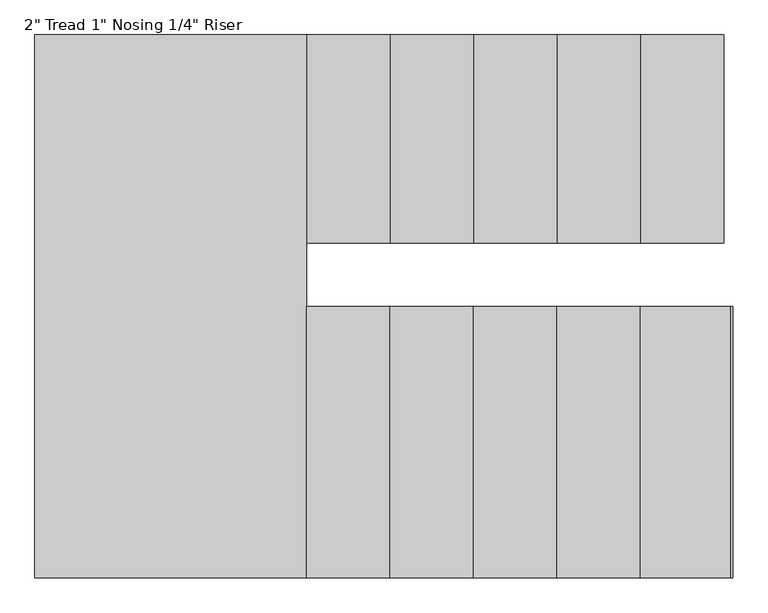
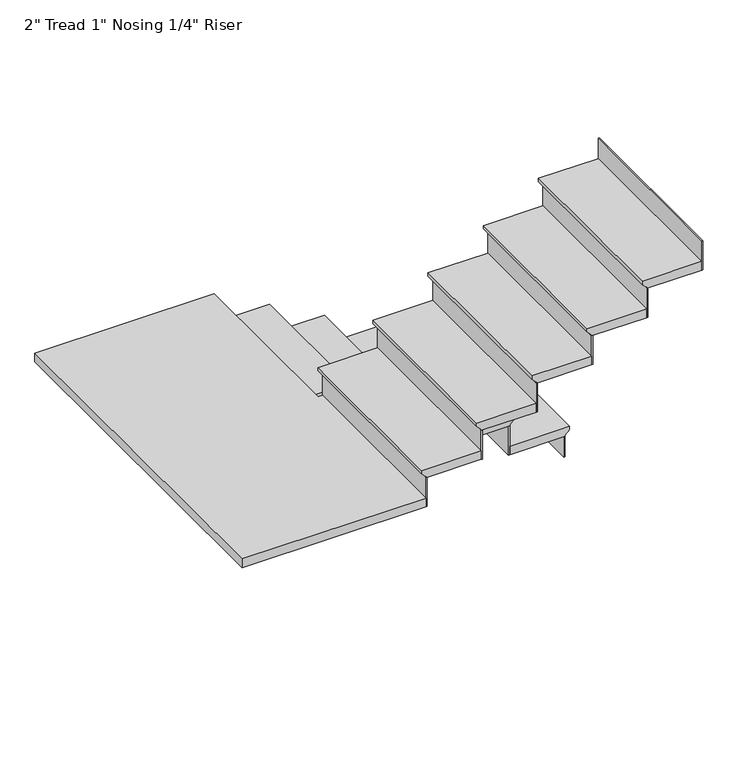
"""IFC4 building model written with IfcOpenShell, lengths in millimetres: stair flight geometry."""

from ifc_helpers import new_model, si_unit, origin, place, context, project, spatial, faceted_brep, source, transform, mapped, element, save


def stair_flight_ed5f4c0f(model_context):
    return source(origin(), model_context, "Body", "Brep", [
        faceted_brep([(-3084.0415084, -317.1427733, 12951.8833333), (-3084.0415084, -317.1427733, 12970.9333333), (-3084.0415084, -1076.6758739, 12970.9333333), (-3084.0415084, -1076.6758739, 12951.8833333), (-3109.4415084, -317.1427733, 12926.4833333), (-3109.4415084, -1076.6758739, 12926.4833333), (-3414.2415084, -317.1427733, 12970.9333333), (-3414.2415084, -1076.6758739, 12970.9333333), (-3109.4415084, -1076.6758739, 12920.1333333), (-3414.2415084, -1076.6758739, 12920.1333333), (-3414.2415084, -317.1427733, 12920.1333333), (-3109.4415084, -317.1427733, 12920.1333333)], [[[0, 1, 2, 3]], [[4, 0, 3, 5]], [[2, 1, 6, 7]], [[8, 9, 10, 11]], [[2, 7, 9, 8, 5, 3]], [[8, 11, 4, 5]], [[6, 1, 0, 4, 11, 10]], [[7, 6, 10, 9]]]),
        faceted_brep([(-3109.4415084, -317.1427733, 12920.1333333), (-3109.4415084, -317.1427733, 12801.6), (-3115.7915084, -317.1427733, 12801.6), (-3115.7915084, -317.1427733, 12920.1333333), (-3109.4415084, -1076.6758739, 12920.1333333), (-3115.7915084, -1076.6758739, 12920.1333333), (-3115.7915084, -1076.6758739, 12801.6), (-3109.4415084, -1076.6758739, 12801.6)], [[[0, 1, 2, 3]], [[4, 5, 6, 7]], [[1, 0, 4, 7]], [[2, 1, 7, 6]], [[3, 2, 6, 5]], [[0, 3, 5, 4]]]),
        faceted_brep([(-3414.2415084, -317.1427733, 13089.4666667), (-3414.2415084, -317.1427733, 12920.1333333), (-3420.5915084, -317.1427733, 12920.1333333), (-3420.5915084, -317.1427733, 13089.4666667), (-3414.2415084, -1076.6758739, 13089.4666667), (-3420.5915084, -1076.6758739, 13089.4666667), (-3420.5915084, -1076.6758739, 12920.1333333), (-3414.2415084, -1076.6758739, 12920.1333333)], [[[0, 1, 2, 3]], [[4, 5, 6, 7]], [[1, 0, 4, 7]], [[2, 1, 7, 6]], [[3, 2, 6, 5]], [[0, 3, 5, 4]]]),
        faceted_brep([(-3388.8415084, -1076.6758739, 13140.2666667), (-3388.8415084, -317.1427733, 13140.2666667), (-3719.0415084, -317.1427733, 13140.2666667), (-3719.0415084, -1076.6758739, 13140.2666667), (-3414.2415084, -1076.6758739, 13089.4666667), (-3719.0415084, -1076.6758739, 13089.4666667), (-3719.0415084, -317.1427733, 13089.4666667), (-3414.2415084, -317.1427733, 13089.4666667), (-3414.2415084, -1076.6758739, 13095.8166667), (-3388.8415084, -1076.6758739, 13121.2166667), (-3414.2415084, -317.1427733, 13095.8166667), (-3388.8415084, -317.1427733, 13121.2166667)], [[[0, 1, 2, 3]], [[4, 5, 6, 7]], [[0, 3, 5, 4, 8, 9]], [[4, 7, 10, 8]], [[2, 1, 11, 10, 7, 6]], [[3, 2, 6, 5]], [[11, 1, 0, 9]], [[10, 11, 9, 8]]]),
        faceted_brep([(-3719.0415084, -317.1427733, 13258.8), (-3719.0415084, -317.1427733, 13089.4666667), (-3725.3915084, -317.1427733, 13089.4666667), (-3725.3915084, -317.1427733, 13258.8), (-3719.0415084, -1076.6758739, 13258.8), (-3725.3915084, -1076.6758739, 13258.8), (-3725.3915084, -1076.6758739, 13089.4666667), (-3719.0415084, -1076.6758739, 13089.4666667)], [[[0, 1, 2, 3]], [[4, 5, 6, 7]], [[1, 0, 4, 7]], [[2, 1, 7, 6]], [[3, 2, 6, 5]], [[0, 3, 5, 4]]]),
        faceted_brep([(-3693.6415084, -1076.6758739, 13309.6), (-3693.6415084, -317.1427733, 13309.6), (-4023.8415084, -317.1427733, 13309.6), (-4023.8415084, -1076.6758739, 13309.6), (-3719.0415084, -1076.6758739, 13258.8), (-4023.8415084, -1076.6758739, 13258.8), (-4023.8415084, -317.1427733, 13258.8), (-3719.0415084, -317.1427733, 13258.8), (-3719.0415084, -1076.6758739, 13265.15), (-3693.6415084, -1076.6758739, 13290.55), (-3719.0415084, -317.1427733, 13265.15), (-3693.6415084, -317.1427733, 13290.55)], [[[0, 1, 2, 3]], [[4, 5, 6, 7]], [[0, 3, 5, 4, 8, 9]], [[4, 7, 10, 8]], [[2, 1, 11, 10, 7, 6]], [[3, 2, 6, 5]], [[11, 1, 0, 9]], [[10, 11, 9, 8]]]),
        faceted_brep([(-4023.8415084, -317.1427733, 13428.1333333), (-4023.8415084, -317.1427733, 13258.8), (-4030.1915084, -317.1427733, 13258.8), (-4030.1915084, -317.1427733, 13428.1333333), (-4023.8415084, -1076.6758739, 13428.1333333), (-4030.1915084, -1076.6758739, 13428.1333333), (-4030.1915084, -1076.6758739, 13258.8), (-4023.8415084, -1076.6758739, 13258.8)], [[[0, 1, 2, 3]], [[4, 5, 6, 7]], [[1, 0, 4, 7]], [[2, 1, 7, 6]], [[3, 2, 6, 5]], [[0, 3, 5, 4]]]),
        faceted_brep([(-3998.4415084, -1076.6758739, 13478.9333333), (-3998.4415084, -317.1427733, 13478.9333333), (-4328.6415084, -317.1427733, 13478.9333333), (-4328.6415084, -1076.6758739, 13478.9333333), (-4023.8415084, -1076.6758739, 13428.1333333), (-4328.6415084, -1076.6758739, 13428.1333333), (-4328.6415084, -317.1427733, 13428.1333333), (-4023.8415084, -317.1427733, 13428.1333333), (-4023.8415084, -1076.6758739, 13434.4833333), (-3998.4415084, -1076.6758739, 13459.8833333), (-4023.8415084, -317.1427733, 13434.4833333), (-3998.4415084, -317.1427733, 13459.8833333)], [[[0, 1, 2, 3]], [[4, 5, 6, 7]], [[0, 3, 5, 4, 8, 9]], [[4, 7, 10, 8]], [[2, 1, 11, 10, 7, 6]], [[3, 2, 6, 5]], [[11, 1, 0, 9]], [[10, 11, 9, 8]]]),
        faceted_brep([(-4328.6415084, -317.1427733, 13597.4666667), (-4328.6415084, -317.1427733, 13428.1333333), (-4334.9915084, -317.1427733, 13428.1333333), (-4334.9915084, -317.1427733, 13597.4666667), (-4328.6415084, -1076.6758739, 13597.4666667), (-4334.9915084, -1076.6758739, 13597.4666667), (-4334.9915084, -1076.6758739, 13428.1333333), (-4328.6415084, -1076.6758739, 13428.1333333)], [[[0, 1, 2, 3]], [[4, 5, 6, 7]], [[1, 0, 4, 7]], [[2, 1, 7, 6]], [[3, 2, 6, 5]], [[0, 3, 5, 4]]]),
        faceted_brep([(-4303.2415084, -1076.6758739, 13648.2666667), (-4303.2415084, -317.1427733, 13648.2666667), (-4633.4415084, -317.1427733, 13648.2666667), (-4633.4415084, -1076.6758739, 13648.2666667), (-4328.6415084, -1076.6758739, 13597.4666667), (-4633.4415084, -1076.6758739, 13597.4666667), (-4633.4415084, -317.1427733, 13597.4666667), (-4328.6415084, -317.1427733, 13597.4666667), (-4328.6415084, -1076.6758739, 13603.8166667), (-4303.2415084, -1076.6758739, 13629.2166667), (-4328.6415084, -317.1427733, 13603.8166667), (-4303.2415084, -317.1427733, 13629.2166667)], [[[0, 1, 2, 3]], [[4, 5, 6, 7]], [[0, 3, 5, 4, 8, 9]], [[4, 7, 10, 8]], [[2, 1, 11, 10, 7, 6]], [[3, 2, 6, 5]], [[11, 1, 0, 9]], [[10, 11, 9, 8]]]),
        faceted_brep([(-4633.4415084, -317.1427733, 13766.8), (-4633.4415084, -317.1427733, 13597.4666667), (-4639.7915084, -317.1427733, 13597.4666667), (-4639.7915084, -317.1427733, 13766.8), (-4633.4415084, -1076.6758739, 13766.8), (-4639.7915084, -1076.6758739, 13766.8), (-4639.7915084, -1076.6758739, 13597.4666667), (-4633.4415084, -1076.6758739, 13597.4666667)], [[[0, 1, 2, 3]], [[4, 5, 6, 7]], [[1, 0, 4, 7]], [[2, 1, 7, 6]], [[3, 2, 6, 5]], [[0, 3, 5, 4]]]),
        faceted_brep([(-4582.6415084, -1307.7427733, 13817.6), (-4608.0415084, -1307.7427733, 13817.6), (-4608.0415084, -317.1427733, 13817.6), (-5598.6415084, -317.1427733, 13817.6), (-5598.6415084, -2298.3427733, 13817.6), (-4582.6415084, -2298.3427733, 13817.6), (-4608.0415084, -1307.7427733, 13766.8), (-4582.6415084, -1307.7427733, 13766.8), (-4582.6415084, -2298.3427733, 13766.8), (-5598.6415084, -2298.3427733, 13766.8), (-5598.6415084, -317.1427733, 13766.8), (-4633.4415084, -317.1427733, 13766.8), (-4633.4415084, -1076.6758739, 13766.8), (-4608.0415084, -1076.6758739, 13766.8), (-4608.0415084, -1076.6758739, 13798.55), (-4608.0415084, -317.1427733, 13798.55), (-4633.4415084, -1076.6758739, 13773.15), (-4633.4415084, -317.1427733, 13773.15)], [[[0, 1, 2, 3, 4, 5]], [[6, 7, 8, 9, 10, 11, 12, 13]], [[1, 0, 7, 6]], [[2, 1, 6, 13, 14, 15]], [[13, 12, 16, 14]], [[12, 11, 17, 16]], [[3, 2, 15, 17, 11, 10]], [[4, 3, 10, 9]], [[5, 4, 9, 8]], [[0, 5, 8, 7]], [[17, 15, 14, 16]]]),
        faceted_brep([(-4582.6415084, -2298.3427733, 13936.1333333), (-4582.6415084, -2298.3427733, 13766.8), (-4576.2915084, -2298.3427733, 13766.8), (-4576.2915084, -2298.3427733, 13936.1333333), (-4582.6415084, -1307.7427733, 13936.1333333), (-4576.2915084, -1307.7427733, 13936.1333333), (-4576.2915084, -1307.7427733, 13766.8), (-4582.6415084, -1307.7427733, 13766.8)], [[[0, 1, 2, 3]], [[4, 5, 6, 7]], [[1, 0, 4, 7]], [[2, 1, 7, 6]], [[3, 2, 6, 5]], [[0, 3, 5, 4]]]),
        faceted_brep([(-4608.0415084, -1307.7427733, 13986.9333333), (-4608.0415084, -2298.3427733, 13986.9333333), (-4277.8415084, -2298.3427733, 13986.9333333), (-4277.8415084, -1307.7427733, 13986.9333333), (-4582.6415084, -1307.7427733, 13936.1333333), (-4277.8415084, -1307.7427733, 13936.1333333), (-4277.8415084, -2298.3427733, 13936.1333333), (-4582.6415084, -2298.3427733, 13936.1333333), (-4582.6415084, -1307.7427733, 13942.4833333), (-4608.0415084, -1307.7427733, 13967.8833333), (-4582.6415084, -2298.3427733, 13942.4833333), (-4608.0415084, -2298.3427733, 13967.8833333)], [[[0, 1, 2, 3]], [[4, 5, 6, 7]], [[0, 3, 5, 4, 8, 9]], [[4, 7, 10, 8]], [[2, 1, 11, 10, 7, 6]], [[3, 2, 6, 5]], [[11, 1, 0, 9]], [[10, 11, 9, 8]]]),
        faceted_brep([(-4277.8415084, -2298.3427733, 14105.4666667), (-4277.8415084, -2298.3427733, 13936.1333333), (-4271.4915084, -2298.3427733, 13936.1333333), (-4271.4915084, -2298.3427733, 14105.4666667), (-4277.8415084, -1307.7427733, 14105.4666667), (-4271.4915084, -1307.7427733, 14105.4666667), (-4271.4915084, -1307.7427733, 13936.1333333), (-4277.8415084, -1307.7427733, 13936.1333333)], [[[0, 1, 2, 3]], [[4, 5, 6, 7]], [[1, 0, 4, 7]], [[2, 1, 7, 6]], [[3, 2, 6, 5]], [[0, 3, 5, 4]]]),
        faceted_brep([(-4303.2415084, -1307.7427733, 14156.2666667), (-4303.2415084, -2298.3427733, 14156.2666667), (-3973.0415084, -2298.3427733, 14156.2666667), (-3973.0415084, -1307.7427733, 14156.2666667), (-4277.8415084, -1307.7427733, 14105.4666667), (-3973.0415084, -1307.7427733, 14105.4666667), (-3973.0415084, -2298.3427733, 14105.4666667), (-4277.8415084, -2298.3427733, 14105.4666667), (-4277.8415084, -1307.7427733, 14111.8166667), (-4303.2415084, -1307.7427733, 14137.2166667), (-4277.8415084, -2298.3427733, 14111.8166667), (-4303.2415084, -2298.3427733, 14137.2166667)], [[[0, 1, 2, 3]], [[4, 5, 6, 7]], [[0, 3, 5, 4, 8, 9]], [[4, 7, 10, 8]], [[2, 1, 11, 10, 7, 6]], [[3, 2, 6, 5]], [[11, 1, 0, 9]], [[10, 11, 9, 8]]]),
        faceted_brep([(-3973.0415084, -2298.3427733, 14274.8), (-3973.0415084, -2298.3427733, 14105.4666667), (-3966.6915084, -2298.3427733, 14105.4666667), (-3966.6915084, -2298.3427733, 14274.8), (-3973.0415084, -1307.7427733, 14274.8), (-3966.6915084, -1307.7427733, 14274.8), (-3966.6915084, -1307.7427733, 14105.4666667), (-3973.0415084, -1307.7427733, 14105.4666667)], [[[0, 1, 2, 3]], [[4, 5, 6, 7]], [[1, 0, 4, 7]], [[2, 1, 7, 6]], [[3, 2, 6, 5]], [[0, 3, 5, 4]]]),
        faceted_brep([(-3998.4415084, -1307.7427733, 14325.6), (-3998.4415084, -2298.3427733, 14325.6), (-3668.2415084, -2298.3427733, 14325.6), (-3668.2415084, -1307.7427733, 14325.6), (-3973.0415084, -1307.7427733, 14274.8), (-3668.2415084, -1307.7427733, 14274.8), (-3668.2415084, -2298.3427733, 14274.8), (-3973.0415084, -2298.3427733, 14274.8), (-3973.0415084, -1307.7427733, 14281.15), (-3998.4415084, -1307.7427733, 14306.55), (-3973.0415084, -2298.3427733, 14281.15), (-3998.4415084, -2298.3427733, 14306.55)], [[[0, 1, 2, 3]], [[4, 5, 6, 7]], [[0, 3, 5, 4, 8, 9]], [[4, 7, 10, 8]], [[2, 1, 11, 10, 7, 6]], [[3, 2, 6, 5]], [[11, 1, 0, 9]], [[10, 11, 9, 8]]]),
        faceted_brep([(-3668.2415084, -2298.3427733, 14444.1333333), (-3668.2415084, -2298.3427733, 14274.8), (-3661.8915084, -2298.3427733, 14274.8), (-3661.8915084, -2298.3427733, 14444.1333333), (-3668.2415084, -1307.7427733, 14444.1333333), (-3661.8915084, -1307.7427733, 14444.1333333), (-3661.8915084, -1307.7427733, 14274.8), (-3668.2415084, -1307.7427733, 14274.8)], [[[0, 1, 2, 3]], [[4, 5, 6, 7]], [[1, 0, 4, 7]], [[2, 1, 7, 6]], [[3, 2, 6, 5]], [[0, 3, 5, 4]]]),
        faceted_brep([(-3693.6415084, -1307.7427733, 14494.9333333), (-3693.6415084, -2298.3427733, 14494.9333333), (-3363.4415084, -2298.3427733, 14494.9333333), (-3363.4415084, -1307.7427733, 14494.9333333), (-3668.2415084, -1307.7427733, 14444.1333333), (-3363.4415084, -1307.7427733, 14444.1333333), (-3363.4415084, -2298.3427733, 14444.1333333), (-3668.2415084, -2298.3427733, 14444.1333333), (-3668.2415084, -1307.7427733, 14450.4833333), (-3693.6415084, -1307.7427733, 14475.8833333), (-3668.2415084, -2298.3427733, 14450.4833333), (-3693.6415084, -2298.3427733, 14475.8833333)], [[[0, 1, 2, 3]], [[4, 5, 6, 7]], [[0, 3, 5, 4, 8, 9]], [[4, 7, 10, 8]], [[2, 1, 11, 10, 7, 6]], [[3, 2, 6, 5]], [[11, 1, 0, 9]], [[10, 11, 9, 8]]]),
        faceted_brep([(-3363.4415084, -2298.3427733, 14613.4666667), (-3363.4415084, -2298.3427733, 14444.1333333), (-3357.0915084, -2298.3427733, 14444.1333333), (-3357.0915084, -2298.3427733, 14613.4666667), (-3363.4415084, -1307.7427733, 14613.4666667), (-3357.0915084, -1307.7427733, 14613.4666667), (-3357.0915084, -1307.7427733, 14444.1333333), (-3363.4415084, -1307.7427733, 14444.1333333)], [[[0, 1, 2, 3]], [[4, 5, 6, 7]], [[1, 0, 4, 7]], [[2, 1, 7, 6]], [[3, 2, 6, 5]], [[0, 3, 5, 4]]]),
        faceted_brep([(-3058.6415084, -2298.3427733, 14782.8), (-3058.6415084, -2298.3427733, 14613.4666667), (-3052.2915084, -2298.3427733, 14613.4666667), (-3052.2915084, -2298.3427733, 14782.8), (-3058.6415084, -1307.7427733, 14782.8), (-3052.2915084, -1307.7427733, 14782.8), (-3052.2915084, -1307.7427733, 14613.4666667), (-3058.6415084, -1307.7427733, 14613.4666667)], [[[0, 1, 2, 3]], [[4, 5, 6, 7]], [[1, 0, 4, 7]], [[2, 1, 7, 6]], [[3, 2, 6, 5]], [[0, 3, 5, 4]]]),
        faceted_brep([(-3388.8415084, -1307.7427733, 14664.2666667), (-3388.8415084, -2298.3427733, 14664.2666667), (-3058.6415084, -2298.3427733, 14664.2666667), (-3058.6415084, -1307.7427733, 14664.2666667), (-3363.4415084, -1307.7427733, 14613.4666667), (-3058.6415084, -1307.7427733, 14613.4666667), (-3058.6415084, -2298.3427733, 14613.4666667), (-3363.4415084, -2298.3427733, 14613.4666667), (-3363.4415084, -1307.7427733, 14619.8166667), (-3388.8415084, -1307.7427733, 14645.2166667), (-3363.4415084, -2298.3427733, 14619.8166667), (-3388.8415084, -2298.3427733, 14645.2166667)], [[[0, 1, 2, 3]], [[4, 5, 6, 7]], [[0, 3, 5, 4, 8, 9]], [[4, 7, 10, 8]], [[2, 1, 11, 10, 7, 6]], [[3, 2, 6, 5]], [[11, 1, 0, 9]], [[10, 11, 9, 8]]]),
    ])


if __name__ == "__main__":
    model = new_model("IFC4")
    model_context = context("Model", 3, world=origin())
    ifc_project = project(units=[si_unit("LENGTHUNIT", "METRE", prefix="MILLI")], contexts=[model_context])
    site = spatial("IfcSite", under=ifc_project)
    building = spatial("IfcBuilding", under=site)
    placement = place(None, origin())
    stair_flight_shape = stair_flight_ed5f4c0f(model_context)
    element("IfcStairFlight", 1, ObjectType="2\" Tread 1\" Nosing 1/4\" Riser", at=placement, inside=building, context=model_context, shape_type="MappedRepresentation", body=[
        mapped(stair_flight_shape, transform((0.0, 0.0, 0.0), x_axis=(1.0, 0.0, 0.0), y_axis=(0.0, 1.0, 0.0), z_axis=(0.0, 0.0, 1.0))),
    ])
    save(model, "model.ifc")
